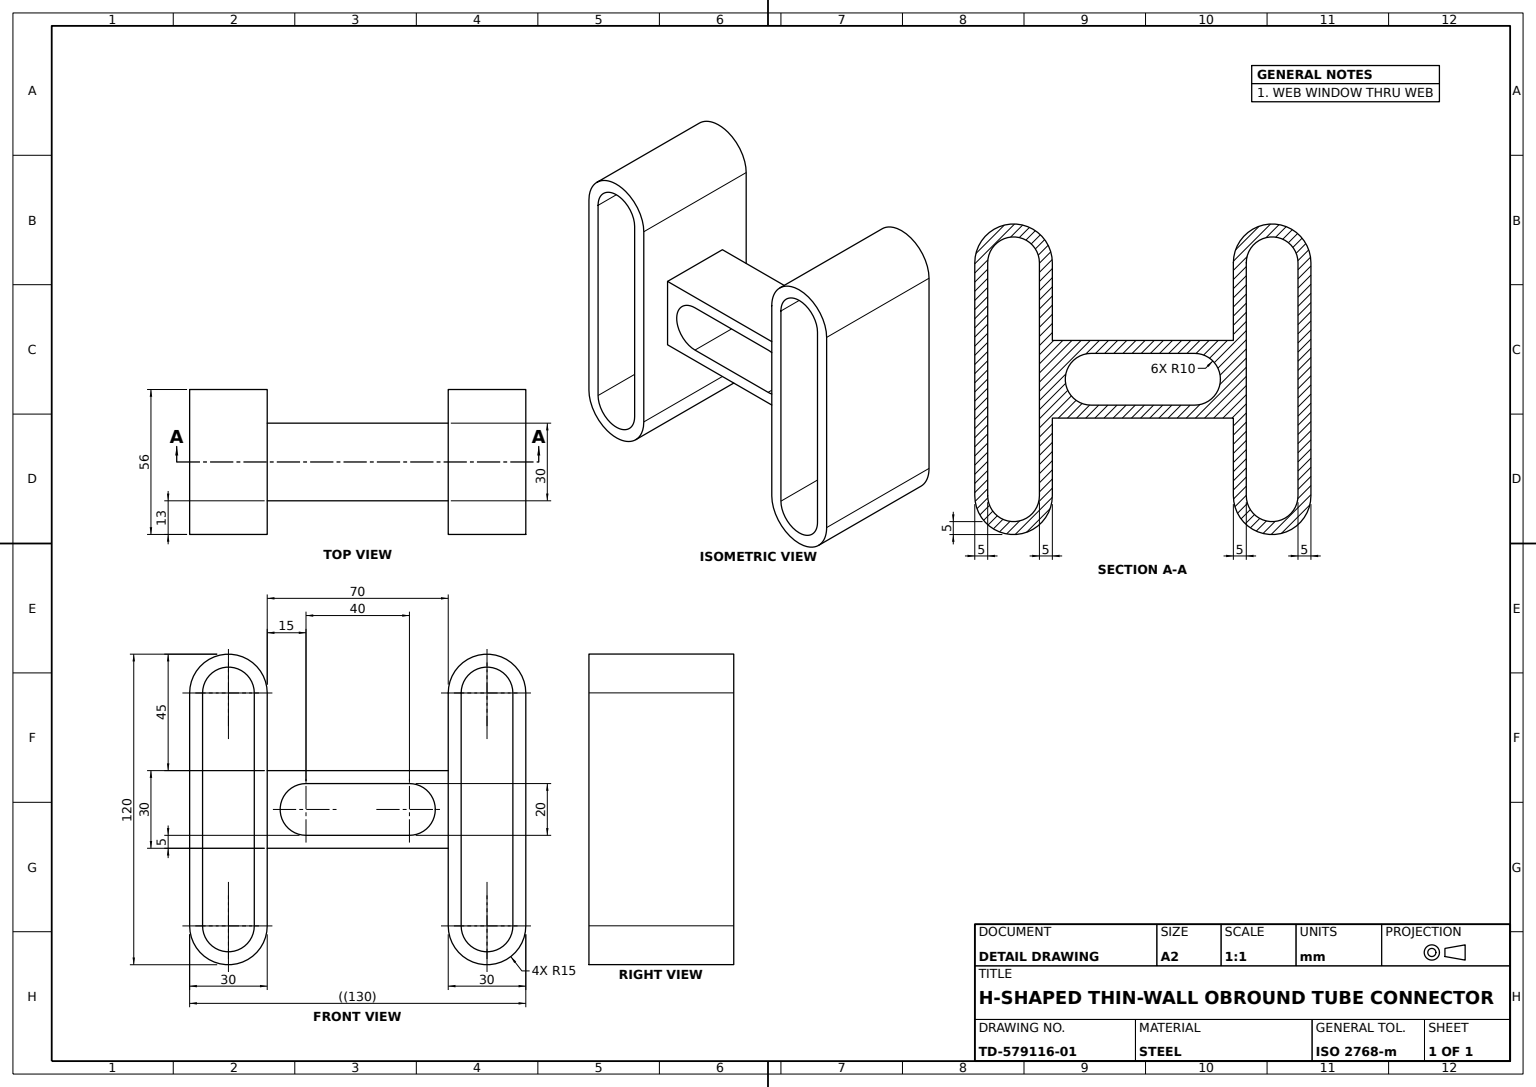
SolidWorks part; units mm, degrees
material "Plain Carbon Steel"
ref_plane "Front Plane" through (0, 0, 0) normal (0, 0, 1) x (1, 0, 0)
ref_plane "Top Plane" through (0, 0, 0) normal (0, 1, 0) x (1, 0, 0)
ref_plane "Right Plane" through (0, 0, 0) normal (1, 0, 0) x (0, 0, -1)
sketch "Center Web Profile" plane through (0, 0, 0) normal (0, 0, 1) x (1, 0, 0)
  line L1 (35, 0) -> (35, 15)
  line L2 (35, 15) -> (-35, 15)
  line L3 (-35, 15) -> (-35, -15)
  line L4 (-35, -15) -> (35, -15)
  line L5 (35, -15) -> (35, 0)
  dimension "D1" = 70
  dimension "D2" = 30
  dimension "D3" = 15
  dimension "D4" = 35
extrude "Center Web" add sketch "Center Web Profile" along normal mid plane 30
sketch "Web Window Profile 40x20" plane through (0, 0, 15) normal (0, 0, 1) x (1, 0, 0)
  line L2 (-20, 10) -> (20, 10)
  line L3 (-20, -10) -> (20, -10)
  arc A0 (20, -10) -> (20, 10) centre (20, 0) ccw
  arc A1 (-20, 10) -> (-20, -10) centre (-20, 0) ccw
  dimension "D1" = 40
  dimension "D2" = 10
  dimension "D3" = 20
  dimension "D4" = 20
extrude "Web Window Cut" cut sketch "Web Window Profile 40x20" against normal blind 80
sketch "Side Loop Profile" plane through (0, 0, 0) normal (0, 0, 1) x (1, 0, 0)
  line L0 (35, 0) -> (35, 45)
  line L1 (35, -15) -> (35, 15) construction
  line L2 (60, 45) -> (60, -45)
  line L3 (65, 45) -> (65, -45)
  line L5 (35, -45) -> (35, -15)
  line L6 (35, -15) -> (35, 0)
  line L7 (40, 45) -> (40, -45)
  arc A0 (65, 45) -> (35, 45) centre (50, 45) ccw
  arc A1 (35, -45) -> (65, -45) centre (50, -45) ccw
  arc A2 (60, 45) -> (40, 45) centre (50, 45) ccw
  arc A3 (40, -45) -> (60, -45) centre (50, -45) ccw
  dimension "D1" = 15
  dimension "D2" = 10
  dimension "D3" = 30
  dimension "D4" = 90
extrude "Side Loop" add sketch "Side Loop Profile" along normal mid plane 56
mirror "Side Loop Mirror" about plane through (0, 0, 0) normal (1, 0, 0) of "Side Loop"
